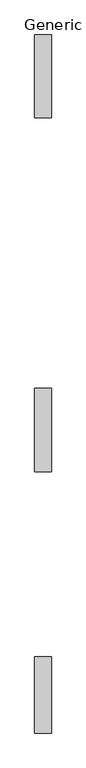
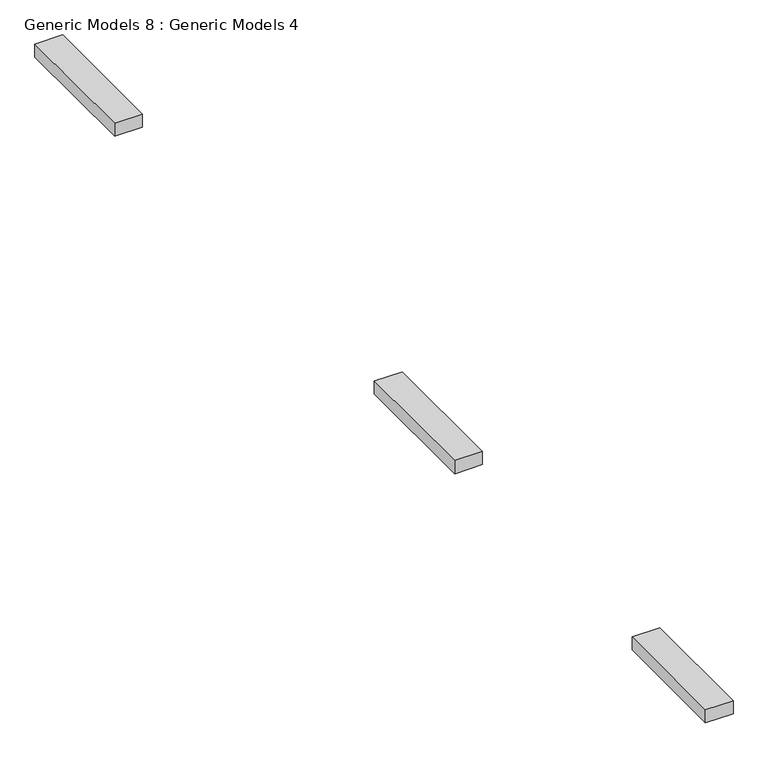
"""IFC4 building model written with IfcOpenShell, lengths in millimetres: proxy geometry, Generic Models 8 : Generic Models 4."""

from ifc_helpers import new_model, si_unit, frame, origin, place, context, project, spatial, polyline, outline, extrude, source, transform, mapped, element, save


def generic_models_8_generic_models_4_251d3b20(model_context):
    return source(origin(), model_context, "Body", "SweptSolid", [
        extrude(outline(polyline([(-15928.6646954, 5920.6374503), (-15928.6646954, 7440.5252636), (-15623.8646954, 7440.5252636), (-15623.8646954, 5920.6374503), (-15928.6646954, 5920.6374503)])), frame((0.0, 0.0, 5613.4), z_axis=(0.0, 0.0, 1.0), x_axis=(1.0, 0.0, 0.0)), (0.0, 0.0, 1.0), 152.4),
        extrude(outline(polyline([(-15928.6646954, -570.5858218), (-15928.6646954, 958.8860888), (-15623.8646954, 958.8860888), (-15623.8646954, -570.5858218), (-15928.6646954, -570.5858218)])), frame((0.0, 0.0, 5613.4), z_axis=(0.0, 0.0, 1.0), x_axis=(1.0, 0.0, 0.0)), (0.0, 0.0, 1.0), 152.4),
        extrude(outline(polyline([(-15928.6646954, -5360.1770128), (-15928.6646954, -3959.3561253), (-15623.8646954, -3959.3561253), (-15623.8646954, -5360.1770128), (-15928.6646954, -5360.1770128)])), frame((0.0, 0.0, 5613.4), z_axis=(0.0, 0.0, 1.0), x_axis=(1.0, 0.0, 0.0)), (0.0, 0.0, 1.0), 152.4),
    ])


if __name__ == "__main__":
    model = new_model("IFC4")
    model_context = context("Model", 3, world=origin())
    ifc_project = project(units=[si_unit("LENGTHUNIT", "METRE", prefix="MILLI")], contexts=[model_context])
    site = spatial("IfcSite", under=ifc_project)
    building = spatial("IfcBuilding", under=site)
    placement = place(None, origin())
    generic_models_8_generic_models_4_shape = generic_models_8_generic_models_4_251d3b20(model_context)
    element("IfcBuildingElementProxy", 1, Name="Generic Models 8 : Generic Models 4", ObjectType="Generic Models 8 : Generic Models 4", at=placement, inside=building, context=model_context, shape_type="MappedRepresentation", body=[
        mapped(generic_models_8_generic_models_4_shape, transform((0.0, 0.0, 0.0), x_axis=(1.0, 0.0, 0.0), y_axis=(0.0, 1.0, 0.0), z_axis=(0.0, 0.0, 1.0))),
    ])
    save(model, "model.ifc")
